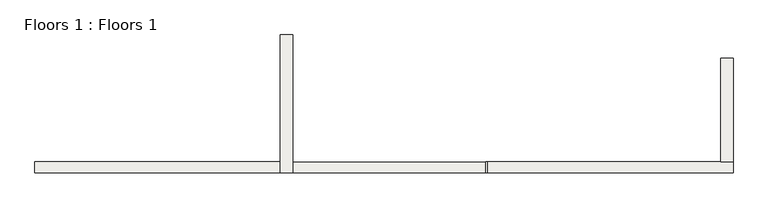
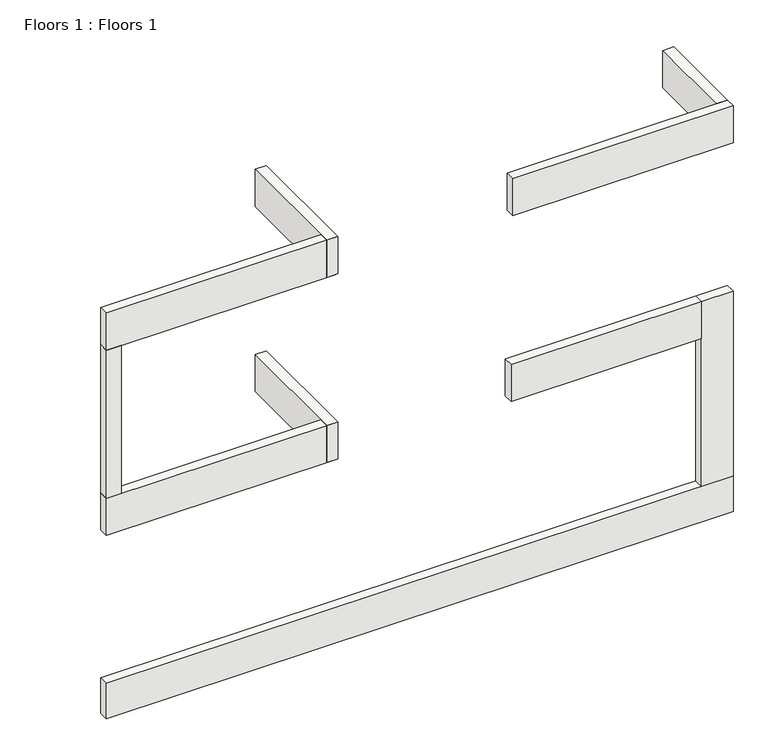
"""IFC4 building model written with IfcOpenShell, lengths in millimetres: slab geometry, Floors 1 : Floors 1."""

from ifc_helpers import new_model, si_unit, frame, origin, place, context, project, spatial, polyline, outline, extrude, source, transform, mapped, element, save


def floors_1_floors_1_452276dc(model_context):
    return source(origin(), model_context, "Body", "SweptSolid", [
        extrude(outline(polyline([(3431.5769214, -622.6464931), (3431.5769214, -2070.4464178), (3258.2721596, -2070.4464178), (3258.2721596, -622.6464931), (3431.5769214, -622.6464931)])), frame((0.0, 0.0, 8534.4), z_axis=(0.0, 0.0, 1.0), x_axis=(1.0, 0.0, 0.0)), (0.0, 0.0, 1.0), 609.6),
        extrude(outline(polyline([(-2719.2279495, -2222.8464178), (-2893.0230786, -2222.8464178), (-2893.0230786, -295.8527599), (-2719.2279495, -295.8527599), (-2719.2279495, -2222.8464178)])), frame((0.0, 0.0, 8534.4), z_axis=(0.0, 0.0, 1.0), x_axis=(1.0, 0.0, 0.0)), (0.0, 0.0, 1.0), 609.6),
        extrude(outline(polyline([(-2719.2279495, -2222.8464178), (-2893.0230786, -2222.8464178), (-2893.0230786, -295.8527599), (-2719.2279495, -295.8527599), (-2719.2279495, -2222.8464178)])), frame((0.0, 0.0, 5486.4), z_axis=(0.0, 0.0, 1.0), x_axis=(1.0, 0.0, 0.0)), (0.0, 0.0, 1.0), 609.6),
        extrude(outline(polyline([(-6093.4230786, -2222.8464178), (-6322.0230786, -2222.8464178), (-6322.0230786, -2070.4464178), (-6093.4230786, -2070.4464178), (-6093.4230786, -2222.8464178)])), frame((0.0, 0.0, 6096.0), z_axis=(0.0, 0.0, 1.0), x_axis=(1.0, 0.0, 0.0)), (0.0, 0.0, 1.0), 2438.4),
        extrude(outline(polyline([(-2791.4230786, -2222.8464178), (-6322.0230786, -2222.8464178), (-6322.0230786, -2070.4464178), (-2791.4230786, -2070.4464178), (-2791.4230786, -2222.8464178)])), frame((0.0, 0.0, 5486.4), z_axis=(0.0, 0.0, 1.0), x_axis=(1.0, 0.0, 0.0)), (0.0, 0.0, 1.0), 609.6),
        extrude(outline(polyline([(3431.5769214, -2222.8464178), (2.5769214, -2222.8464178), (2.5769214, -2070.4464178), (3431.5769214, -2070.4464178), (3431.5769214, -2222.8464178)])), frame((0.0, 0.0, 8534.4), z_axis=(0.0, 0.0, 1.0), x_axis=(1.0, 0.0, 0.0)), (0.0, 0.0, 1.0), 609.6),
        extrude(outline(polyline([(-2750.0780257, -2222.8464178), (-6322.0230786, -2222.8464178), (-6322.0230786, -2070.4464178), (-2750.0780257, -2070.4464178), (-2750.0780257, -2222.8464178)])), frame((0.0, 0.0, 8534.4), z_axis=(0.0, 0.0, 1.0), x_axis=(1.0, 0.0, 0.0)), (0.0, 0.0, 1.0), 609.6),
        extrude(outline(polyline([(2937.7703602, -2222.8464178), (-22.6504261, -2222.8464178), (-22.6504261, -2070.4464178), (2937.7703602, -2070.4464178), (2937.7703602, -2222.8464178)])), frame((0.0, 0.0, 5486.4), z_axis=(0.0, 0.0, 1.0), x_axis=(1.0, 0.0, 0.0)), (0.0, 0.0, 1.0), 609.6),
        extrude(outline(polyline([(3431.5769214, -2222.8464178), (2937.7703602, -2222.8464178), (2937.7703602, -2070.4464178), (3431.5769214, -2070.4464178), (3431.5769214, -2222.8464178)])), frame((0.0, 0.0, 3048.0), z_axis=(0.0, 0.0, 1.0), x_axis=(1.0, 0.0, 0.0)), (0.0, 0.0, 1.0), 3048.0),
        extrude(outline(polyline([(3431.5769214, -2222.8464178), (-6322.0230786, -2222.8464178), (-6322.0230786, -2070.4464178), (3431.5769214, -2070.4464178), (3431.5769214, -2222.8464178)])), frame((0.0, 0.0, 2463.8), z_axis=(0.0, 0.0, 1.0), x_axis=(1.0, 0.0, 0.0)), (0.0, 0.0, 1.0), 584.2),
    ])


if __name__ == "__main__":
    model = new_model("IFC4")
    model_context = context("Model", 3, world=origin())
    ifc_project = project(units=[si_unit("LENGTHUNIT", "METRE", prefix="MILLI")], contexts=[model_context])
    site = spatial("IfcSite", under=ifc_project)
    building = spatial("IfcBuilding", under=site)
    placement = place(None, origin())
    floors_1_floors_1_shape = floors_1_floors_1_452276dc(model_context)
    element("IfcSlab", 1, ObjectType="Floors 1 : Floors 1", at=placement, inside=building, context=model_context, shape_type="MappedRepresentation", body=[
        mapped(floors_1_floors_1_shape, transform((0.0, 0.0, 0.0), x_axis=(1.0, 0.0, 0.0), y_axis=(0.0, 1.0, 0.0), z_axis=(0.0, 0.0, 1.0))),
    ])
    save(model, "model.ifc")

# Revit data of these elements
# Element 1 (IfcSlab, "Floors 1 : Floors 1")
#   Materials on its faces: "Default Floor", "1 wall"
# Materials
#   "Default Floor": colour RGB 128 128 128, transparency 0, Cost = 0
#   "1 wall": class "Generic", colour RGB 244 245 241, transparency 0, Cost = 0
